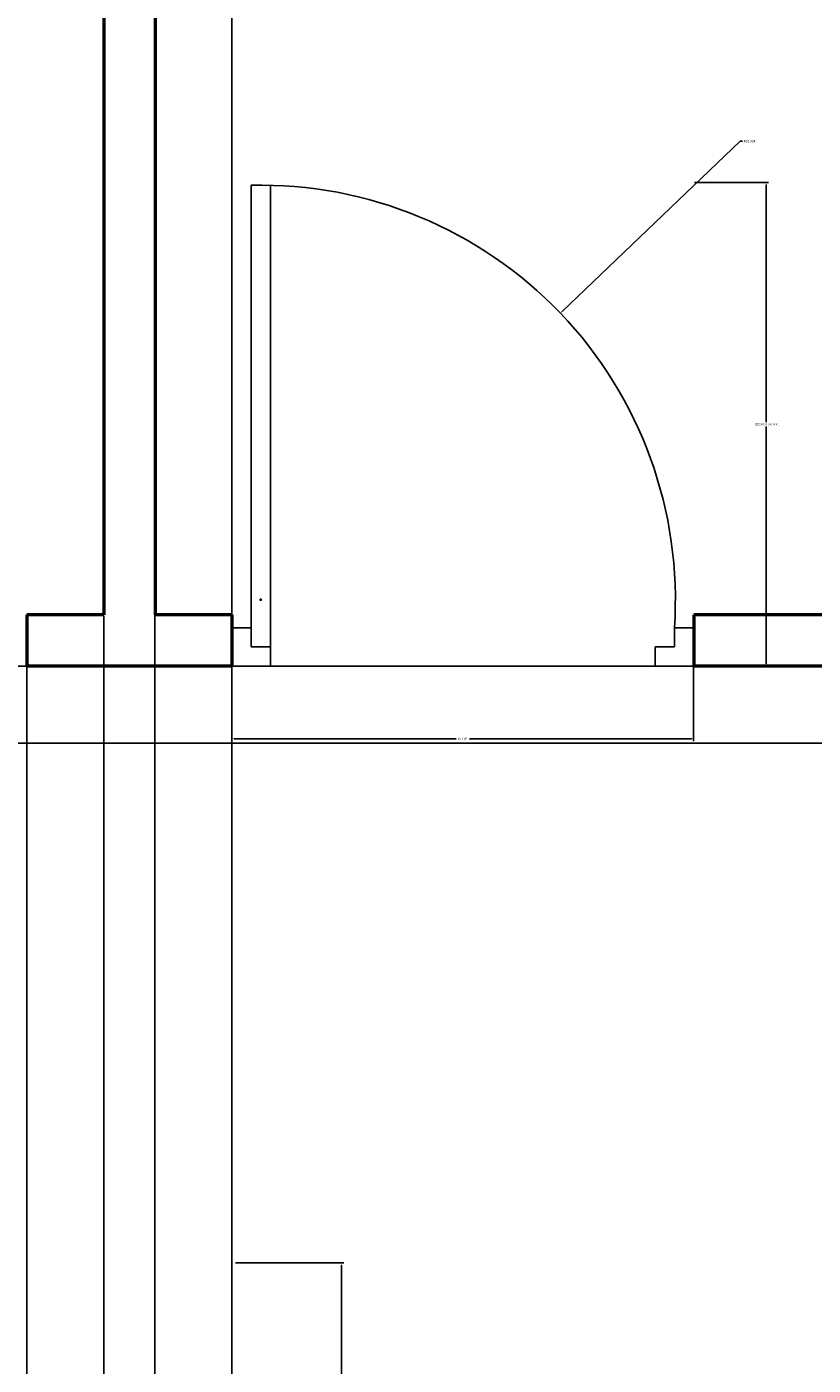
# Model space of a CAD drawing. Units: inches. Extents: x 1798 to 2141, y 1923 to 2386.
# Tile 7 of 9: x 1967 to 2028, y 2177 to 2281. Entities that reach past the tile are written whole.
import ezdxf

# ---------------------------------------------------------------- set-up
doc = ezdxf.new("R2010")
doc.units = ezdxf.units.IN
for name, color, linetype, lineweight in [('A-ANNO-DIMS', 2, 'Continuous', 18), ('A-FURN', 8, 'Continuous', 13), ('door', 40, 'Continuous', 25), ('wall', 4, 'Continuous', 50)]:
    doc.layers.add(name, color=color, linetype=linetype, lineweight=lineweight)
doc.styles.get("Standard").update_dxf_attribs({"font": 'arial.ttf'})
doc.dimstyles.get("Standard").update_dxf_attribs({"dimtxt": 0.18, "dimasz": 0.18, "dimexe": 0.18, "dimexo": 0.0625, "dimgap": 0.09, "dimtad": 0, "dimtih": 1, "dimtoh": 1, "dimdec": 4, "dimzin": 0, "dimdsep": 46, "dimtxsty": 'Standard', "dimcen": 0.09, "dimadec": 0, "dimazin": 0, "dimtfac": 1, "dimtdec": 4, "dimtofl": 0, "dimtmove": 0, "dimatfit": 3, "dimfxl": 1, "dimtolj": 1, "dimtzin": 0, "dimarcsym": 0})

# ---------------------------------------------------------------- blocks, each defined once
blk = doc.blocks.new('A$C45501D90')
for p, q in [((-242.2, 1133.5), (224, 1133.5)), ((-242.2, 1112.8), (-242.2, 1133.5)), ((224, 1112.8), (-242.2, 1112.8)), ((-242.2, 1111.2), (-202.3, 1079.2)), ((-156, 1109.6), (-132, 1085.6)), ((-108.1, 1109.6), (-84.1, 1085.6)), ((-60.2, 1109.6), (-36.2, 1085.6)), ((45.2, 1109.6), (21.2, 1085.6)), ((93.1, 1109.6), (69.1, 1085.6)), ((141, 1109.6), (117, 1085.6)), ((224, 1112.8), (187.3, 1079.2)), ((224, 1133.5), (224, 1112.8)), ((-203.9, 1106.4), (-165.6, 1108)), ((-168.8, 1080.8), (-203.9, 1106.4)), ((-202.3, 1079.2), (-168.8, 1080.8)), ((161.8, 1076.1), (-181.4, 1076.1)), ((-165.6, 1108), (-167.2, 1085.6)), ((-119.3, 1085.6), (-143.2, 1108)), ((-143.2, 1108), (-133.6, 1108)), ((-133.6, 1108), (-122.5, 1098.4)), ((-132, 1085.6), (-119.3, 1085.6)), ((-122.5, 1098.4), (-119.3, 1101.6)), ((-119.3, 1101.6), (-117.7, 1087.2)), ((-71.4, 1085.6), (-95.3, 1108)), ((-95.3, 1108), (-85.7, 1108)), ((-85.7, 1108), (-74.6, 1098.4)), ((-84.1, 1085.6), (-71.4, 1085.6)), ((-74.6, 1098.4), (-71.4, 1101.6)), ((-71.4, 1101.6), (-69.8, 1087.2)), ((-23.5, 1085.6), (-47.4, 1108)), ((-47.4, 1108), (-37.8, 1108)), ((-37.8, 1108), (-26.7, 1098.4)), ((-36.2, 1085.6), (-23.5, 1085.6)), ((-26.7, 1098.4), (-23.5, 1101.6)), ((-23.5, 1101.6), (-21.9, 1087.2)), ((8.5, 1101.6), (6.9, 1087.2)), ((8.5, 1085.6), (32.4, 1108)), ((11.6, 1098.4), (8.5, 1101.6)), ((21.2, 1085.6), (8.5, 1085.6)), ((22.8, 1108), (11.6, 1098.4)), ((32.4, 1108), (22.8, 1108)), ((56.3, 1101.6), (54.8, 1087.2)), ((56.3, 1085.6), (80.3, 1108)), ((59.5, 1098.4), (56.3, 1101.6)), ((69.1, 1085.6), (56.3, 1085.6)), ((70.7, 1108), (59.5, 1098.4)), ((80.3, 1108), (70.7, 1108)), ((104.2, 1101.6), (102.6, 1087.2)), ((104.2, 1085.6), (128.2, 1108)), ((107.4, 1098.4), (104.2, 1101.6)), ((117, 1085.6), (104.2, 1085.6)), ((118.6, 1108), (107.4, 1098.4)), ((128.2, 1108), (118.6, 1108)), ((188.9, 1106.4), (150.5, 1108)), ((150.5, 1108), (152.1, 1085.6)), ((153.7, 1080.8), (188.9, 1106.4)), ((187.3, 1079.2), (153.7, 1080.8)), ((-197.3, 1061.6), (-238.9, 627.6)), ((225.2, 627.8), (177.6, 1061.8)), ((842.6, 766.1), (860.5, 776.5)), ((860.5, 776.5), (1093.6, 372.8)), ((-1102.7, 357), (-869.7, 760.7)), ((-851.7, 750.4), (-1084.8, 346.6)), ((-869.7, 760.7), (-851.7, 750.4)), ((-848.7, 752.3), (-841, 701.8)), ((841.2, 765.3), (833.5, 714.8)), ((1075.7, 362.4), (842.6, 766.1)), ((851.7, 686.6), (856.2, 729.8)), ((856.2, 729.8), (876.7, 697.4)), ((-863.7, 716.7), (-884.3, 684.4)), ((-884.3, 684.4), (-864.1, 674.6)), ((-859.2, 673.6), (-863.7, 716.7)), ((-841, 701.8), (-859.2, 673.6)), ((-431.1, 509), (-830.8, 684.8)), ((820.7, 701.7), (424.1, 520.7)), ((833.5, 714.8), (851.7, 686.6)), ((1012.8, 397.9), (841.2, 695.1)), ((876.7, 697.4), (856.6, 687.6)), ((882.9, 689.9), (874.2, 657.2)), ((-851, 678.1), (-1022.6, 380.9)), ((-897.5, 642.2), (-901.9, 641.1)), ((-901.9, 641.1), (-890.2, 632.5)), ((-895.4, 665), (-900.2, 656.7)), ((-900.2, 656.7), (-897.5, 642.2)), ((-888.1, 633.1), (-895.4, 665)), ((-890.4, 676.9), (-881.7, 644.2)), ((-881.7, 644.2), (-888.1, 633.1)), ((874.2, 657.2), (880.6, 646.1)), ((880.6, 646.1), (887.9, 678)), ((894.4, 654.1), (882.7, 645.5)), ((887.9, 678), (892.7, 669.7)), ((892.7, 669.7), (890, 655.2)), ((890, 655.2), (894.4, 654.1)), ((906.9, 648.4), (898.1, 615.7)), ((-921.5, 600.8), (-925.8, 599.6)), ((-925.8, 599.6), (-914.2, 591)), ((-919.4, 623.5), (-924.2, 615.2)), ((-924.2, 615.2), (-921.5, 600.8)), ((-912, 591.6), (-919.4, 623.5)), ((-914.4, 635.4), (-905.6, 602.7)), ((-905.6, 602.7), (-912, 591.6)), ((-223, 610.1), (209.4, 610.1)), ((898.1, 615.7), (904.5, 604.6)), ((904.5, 604.6), (911.9, 636.5)), ((918.3, 612.6), (906.7, 604)), ((911.9, 636.5), (916.7, 628.2)), ((916.7, 628.2), (914, 613.8)), ((914, 613.8), (918.3, 612.6)), ((930.8, 606.9), (922.1, 574.2)), ((-945.4, 559.3), (-949.8, 558.1)), ((-949.8, 558.1), (-938.1, 549.6)), ((-943.3, 582), (-948.1, 573.8)), ((-948.1, 573.8), (-945.4, 559.3)), ((-936, 550.1), (-943.3, 582)), ((-938.3, 593.9), (-929.6, 561.2)), ((-929.6, 561.2), (-936, 550.1)), ((922.1, 574.2), (928.4, 563.1)), ((928.4, 563.1), (935.8, 595.1)), ((942.3, 571.1), (930.6, 562.6)), ((935.8, 595.1), (940.6, 586.8)), ((940.6, 586.8), (937.9, 572.3)), ((937.9, 572.3), (942.3, 571.1)), ((-951.9, 522.5), (-983.2, 512.9)), ((-983.2, 512.9), (-978.5, 521.2)), ((-978.5, 521.2), (-964.6, 526.1)), ((-964.6, 526.1), (-965.7, 530.5)), ((-965.7, 530.5), (-952.5, 524.7)), ((-958.3, 511.4), (-951.9, 522.5)), ((950.8, 524.4), (944.4, 535.5)), ((944.4, 535.5), (975.7, 525.9)), ((958.2, 543.5), (945, 537.7)), ((983.5, 515.7), (950.8, 524.4)), ((957.1, 539.1), (958.2, 543.5)), ((970.9, 534.2), (957.1, 539.1)), ((975.7, 525.9), (970.9, 534.2)), ((-1015, 461.2), (-982.3, 469.9)), ((-975.9, 481), (-1007.2, 471.4)), ((-1007.2, 471.4), (-1002.4, 479.7)), ((-1002.4, 479.7), (-988.5, 484.6)), ((-991, 502.7), (-958.3, 511.4)), ((-988.5, 484.6), (-989.7, 489)), ((-989.7, 489), (-976.5, 483.2)), ((-982.3, 469.9), (-975.9, 481)), ((-639.9, 111.9), (-423.7, 486.4)), ((-5.6, 508.7, 90.8), (0.4, 508.7, 90.8)), ((-5.6, 317.7, 90.8), (-5.6, 508.7, 90.8)), ((0.4, 508.7, 90.8), (0.4, 317.7, 90.8)), ((5.8, 317.7, 90.8), (5.8, 508.7, 90.8)), ((5.8, 508.7, 90.8), (11.8, 508.7, 90.8)), ((11.8, 508.7, 90.8), (11.8, 317.7, 90.8)), ((416.9, 498.2), (633.1, 123.7)), ((968.4, 494), (999.7, 484.4)), ((974.7, 483), (968.4, 494)), ((982.2, 502), (968.9, 496.2)), ((1007.4, 474.2), (974.7, 483)), ((981, 497.6), (982.2, 502)), ((994.9, 492.7), (981, 497.6)), ((999.7, 484.4), (994.9, 492.7)), ((-1038.9, 419.7), (-1006.2, 428.5)), ((-999.8, 439.5), (-1031.1, 430)), ((-1031.1, 430), (-1026.3, 438.3)), ((-1026.3, 438.3), (-1012.5, 443.1)), ((-1012.5, 443.1), (-1013.6, 447.5)), ((-1013.6, 447.5), (-1000.4, 441.7)), ((-1006.2, 428.5), (-999.8, 439.5)), ((998.7, 441.5), (992.3, 452.5)), ((992.3, 452.5), (1023.6, 443)), ((1006.1, 460.5), (992.9, 454.7)), ((1031.4, 432.7), (998.7, 441.5)), ((1005, 456.2), (1006.1, 460.5)), ((1018.8, 451.3), (1005, 456.2)), ((1023.6, 443), (1018.8, 451.3)), ((-1060.1, 376.6), (-1042.3, 410.6)), ((-1020.4, 394.3), (-1060.1, 376.6)), ((-1042.3, 410.6), (-1023.8, 398.1)), ((-1035.8, 364.4), (-1020.4, 394.3)), ((1028.3, 377.5), (1012.9, 407.3)), ((1012.9, 407.3), (1052.6, 389.6)), ((1034.8, 423.6), (1016.3, 411.1)), ((1052.6, 389.6), (1034.8, 423.6)), ((-1084.8, 346.6), (-1102.7, 357)), ((-1083.4, 345.8), (-1035.8, 364.4)), ((-1018, 360), (-663, 106.9)), ((-22.3, 329.1, 90.8), (-22.3, 344.6, 90.8)), ((-22.3, 344.6, 90.8), (-5.6, 344.6, 90.8)), ((0.4, 344.6, 90.8), (5.8, 344.6, 90.8)), ((11.8, 344.6, 90.8), (27.3, 344.6, 90.8)), ((27.3, 344.6, 90.8), (27.3, 329.1, 90.8)), ((656.3, 118.9), (1008.4, 377.1)), ((1075.9, 358.8), (1028.3, 377.5)), ((1093.6, 372.8), (1075.7, 362.4)), ((-5.6, 329.1, 90.8), (-22.3, 329.1, 90.8)), ((0.4, 317.7, 90.8), (-5.6, 317.7, 90.8)), ((5.8, 329.1, 90.8), (0.4, 329.1, 90.8)), ((11.8, 317.7, 90.8), (5.8, 317.7, 90.8)), ((27.3, 329.1, 90.8), (11.8, 329.1, 90.8)), ((-436.3, 265.3, 90.8), (-433.3, 270.5, 90.8)), ((-270.9, 169.9, 90.8), (-436.3, 265.3, 90.8)), ((-433.3, 270.5, 90.8), (-267.9, 175, 90.8)), ((-430.6, 275.2, 90.8), (-427.6, 280.3, 90.8)), ((-265.2, 179.7, 90.8), (-430.6, 275.2, 90.8)), ((-427.6, 280.3, 90.8), (-262.3, 184.9, 90.8)), ((-175.3, 276.1, 90.8), (-104.8, 293.2, 90.8)), ((-103.3, 252.4, 90.8), (-175.3, 276.1, 90.8)), ((-104.8, 293.2, 90.8), (-85.5, 278.4, 90.8)), ((-85.5, 278.4, 90.8), (-52.1, 293.9, 90.8)), ((9.5, 276.1, 90.8), (-59.5, 246.5, 90.8)), ((-52.1, 293.9, 90.8), (9.5, 276.1, 90.8)), ((134.3, 288, 90.8), (184.3, 235.5, 90.8)), ((149.7, 213.9, 90.8), (134.3, 288, 90.8)), ((255.2, 161.9, 90.8), (420.6, 257.3, 90.8)), ((420.6, 257.3, 90.8), (423.5, 252.2, 90.8)), ((-59.5, 246.5, 90.8), (-103.3, 252.4, 90.8)), ((166.5, 173, 90.8), (149.7, 213.9, 90.8)), ((184.3, 235.5, 90.8), (181.1, 211.4, 90.8)), ((423.5, 252.2, 90.8), (258.2, 156.7, 90.8)), ((260.9, 152, 90.8), (426.2, 247.5, 90.8)), ((429.2, 242.3, 90.8), (263.8, 146.9, 90.8)), ((426.2, 247.5, 90.8), (429.2, 242.3, 90.8)), ((-302.5, 168.8, 90.8), (-294.2, 183.3, 90.8)), ((-291.2, 188.5, 90.8), (-288.5, 193.1, 90.8)), ((-280.7, 175.5, 90.8), (-289.1, 161.1, 90.8)), ((-285.5, 198.3, 90.8), (-277.8, 211.7, 90.8)), ((-277.8, 211.7, 90.8), (-264.3, 204, 90.8)), ((-275.1, 185.4, 90.8), (-277.8, 180.7, 90.8)), ((-264.3, 204, 90.8), (-272.1, 190.5, 90.8)), ((-267.9, 175, 90.8), (-270.9, 169.9, 90.8)), ((-262.3, 184.9, 90.8), (-265.2, 179.7, 90.8)), ((226.7, 128.1, 90.8), (166.5, 173, 90.8)), ((181.1, 211.4, 90.8), (211.3, 190.3, 90.8)), ((211.3, 190.3, 90.8), (226.7, 128.1, 90.8)), ((256.6, 182, 90.8), (270.1, 189.8, 90.8)), ((265, 167.5, 90.8), (256.6, 182, 90.8)), ((270.1, 189.8, 90.8), (278.4, 175.3, 90.8)), ((-289.1, 161.1, 90.8), (-302.5, 168.8, 90.8)), ((-273.6, 117.6, 90.8), (-227.4, 162.1, 90.8)), ((-227.4, 162.1, 90.8), (-236.2, 87.5, 90.8)), ((258.2, 156.7, 90.8), (255.2, 161.9, 90.8)), ((263.8, 146.9, 90.8), (260.9, 152, 90.8)), ((270.7, 157.7, 90.8), (268, 162.4, 90.8)), ((281.4, 139.1, 90.8), (273.7, 152.5, 90.8)), ((281.4, 170.1, 90.8), (284.1, 165.5, 90.8)), ((294.9, 146.8, 90.8), (281.4, 139.1, 90.8)), ((287.1, 160.3, 90.8), (294.9, 146.8, 90.8)), ((-276.8, 80.9, 90.8), (-273.6, 117.6, 90.8)), ((-236.2, 87.5, 90.8), (-263.2, 52.5, 90.8)), ((-319.8, 2.1, 90.8), (-299.3, 71.7, 90.8)), ((-263.2, 52.5, 90.8), (-319.8, 2.1, 90.8)), ((-299.3, 71.7, 90.8), (-276.8, 80.9, 90.8)), ((242.9, -24.6, 90.8), (299.4, 25.9, 90.8)), ((299.4, 25.9, 90.8), (278.9, -43.7, 90.8)), ((215.8, -59.5, 90.8), (242.9, -24.6, 90.8)), ((207, -134.1, 90.8), (215.8, -59.5, 90.8)), ((256.4, -53, 90.8), (253.2, -89.7, 90.8)), ((278.9, -43.7, 90.8), (256.4, -53, 90.8)), ((-656.3, -118.9), (-1008.4, -377.1)), ((-416.9, -498.2), (-633.1, -123.7)), ((-449.6, -214.4, 90.8), (-284.2, -118.9, 90.8)), ((-281.2, -124.1, 90.8), (-446.6, -219.5, 90.8)), ((-315.2, -118.9, 90.8), (-301.8, -111.1, 90.8)), ((-307.5, -132.3, 90.8), (-315.2, -118.9, 90.8)), ((-301.8, -111.1, 90.8), (-294, -124.6, 90.8)), ((-284.2, -118.9, 90.8), (-281.2, -124.1, 90.8)), ((-247, -100.1, 90.8), (-186.8, -145, 90.8)), ((-231.7, -162.3, 90.8), (-247, -100.1, 90.8)), ((253.2, -89.7, 90.8), (207, -134.1, 90.8)), ((639.9, -111.9), (423.7, -486.4)), ((1018, -360), (663, -106.9)), ((-443.9, -224.2, 90.8), (-278.5, -128.7, 90.8)), ((-275.5, -133.9, 90.8), (-440.9, -229.4, 90.8)), ((-301.8, -142.1, 90.8), (-304.5, -137.5, 90.8)), ((-290.4, -161.8, 90.8), (-298.8, -147.3, 90.8)), ((-291, -129.7, 90.8), (-288.3, -134.4, 90.8)), ((-277, -154, 90.8), (-290.4, -161.8, 90.8)), ((-285.4, -139.5, 90.8), (-277, -154, 90.8)), ((-278.5, -128.7, 90.8), (-275.5, -133.9, 90.8)), ((-201.5, -183.4, 90.8), (-231.7, -162.3, 90.8)), ((-186.8, -145, 90.8), (-170.1, -185.9, 90.8)), ((241.9, -156.9, 90.8), (244.9, -151.7, 90.8)), ((407.3, -252.4, 90.8), (241.9, -156.9, 90.8)), ((244, -176, 90.8), (251.7, -162.5, 90.8)), ((244.9, -151.7, 90.8), (410.3, -247.2, 90.8)), ((247.6, -147.1, 90.8), (250.6, -141.9, 90.8)), ((413, -242.5, 90.8), (247.6, -147.1, 90.8)), ((250.6, -141.9, 90.8), (415.9, -237.4, 90.8)), ((254.7, -157.4, 90.8), (257.4, -152.7, 90.8)), ((265.2, -170.3, 90.8), (257.4, -183.7, 90.8)), ((260.4, -147.6, 90.8), (268.7, -133.1, 90.8)), ((270.8, -160.5, 90.8), (268.1, -165.1, 90.8)), ((268.7, -133.1, 90.8), (282.2, -140.8, 90.8)), ((282.2, -140.8, 90.8), (273.8, -155.3, 90.8)), ((-204.7, -207.6, 90.8), (-201.5, -183.4, 90.8)), ((-154.7, -260.1, 90.8), (-204.7, -207.6, 90.8)), ((-170.1, -185.9, 90.8), (-154.7, -260.1, 90.8)), ((257.4, -183.7, 90.8), (244, -176, 90.8)), ((-446.6, -219.5, 90.8), (-449.6, -214.4, 90.8)), ((-440.9, -229.4, 90.8), (-443.9, -224.2, 90.8)), ((-29.8, -248.2, 90.8), (39.2, -218.5, 90.8)), ((31.8, -266, 90.8), (-29.8, -248.2, 90.8)), ((65.2, -250.4, 90.8), (31.8, -266, 90.8)), ((39.2, -218.5, 90.8), (83, -224.4, 90.8)), ((84.4, -265.2, 90.8), (65.2, -250.4, 90.8)), ((83, -224.4, 90.8), (154.9, -248.2, 90.8)), ((154.9, -248.2, 90.8), (84.4, -265.2, 90.8)), ((410.3, -247.2, 90.8), (407.3, -252.4, 90.8)), ((415.9, -237.4, 90.8), (413, -242.5, 90.8)), ((-32.1, -480.7, 90.8), (-32.1, -289.8, 90.8)), ((-32.1, -289.8, 90.8), (-26.1, -289.8, 90.8)), ((-26.1, -289.8, 90.8), (-26.1, -480.7, 90.8)), ((-20.8, -480.7, 90.8), (-20.8, -289.8, 90.8)), ((-20.8, -289.8, 90.8), (-14.8, -289.8, 90.8)), ((-14.8, -289.8, 90.8), (-14.8, -480.7, 90.8)), ((-47.6, -316.6, 90.8), (-47.6, -301.1, 90.8)), ((-47.6, -301.1, 90.8), (-32.1, -301.1, 90.8)), ((-32.1, -316.6, 90.8), (-47.6, -316.6, 90.8)), ((-26.1, -301.1, 90.8), (-20.8, -301.1, 90.8)), ((-20.8, -316.6, 90.8), (-26.1, -316.6, 90.8)), ((-14.8, -301.1, 90.8), (1.9, -301.1, 90.8)), ((1.9, -316.6, 90.8), (-14.8, -316.6, 90.8)), ((1.9, -301.1, 90.8), (1.9, -316.6, 90.8)), ((-1093.6, -372.8), (-1075.7, -362.4)), ((-860.5, -776.5), (-1093.6, -372.8)), ((-1075.9, -358.8), (-1028.3, -377.5)), ((-1075.7, -362.4), (-842.6, -766.1)), ((-1028.3, -377.5), (-1012.9, -407.3)), ((851, -678.1), (1022.6, -380.9)), ((851.7, -750.4), (1084.8, -346.6)), ((1102.7, -357), (869.7, -760.7)), ((1035.8, -364.4), (1020.4, -394.3)), ((1020.4, -394.3), (1060.1, -376.6)), ((1083.4, -345.8), (1035.8, -364.4)), ((1060.1, -376.6), (1042.3, -410.6)), ((1084.8, -346.6), (1102.7, -357)), ((-1052.6, -389.6), (-1034.8, -423.6)), ((-1012.9, -407.3), (-1052.6, -389.6)), ((-1034.8, -423.6), (-1016.3, -411.1)), ((-1012.8, -397.9), (-841.2, -695.1)), ((1038.9, -419.7), (1006.2, -428.5)), ((1042.3, -410.6), (1023.8, -398.1)), ((-1031.4, -432.7), (-998.7, -441.5)), ((-1023.6, -443), (-1018.8, -451.3)), ((-992.3, -452.5), (-1023.6, -443)), ((-1018.8, -451.3), (-1005, -456.2)), ((-1006.1, -460.5), (-992.9, -454.7)), ((-1005, -456.2), (-1006.1, -460.5)), ((-998.7, -441.5), (-992.3, -452.5)), ((1015, -461.2), (982.3, -469.9)), ((1006.2, -428.5), (999.8, -439.5)), ((999.8, -439.5), (1031.1, -430)), ((1013.6, -447.5), (1000.4, -441.7)), ((1026.3, -438.3), (1012.5, -443.1)), ((1012.5, -443.1), (1013.6, -447.5)), ((1031.1, -430), (1026.3, -438.3)), ((-1007.4, -474.2), (-974.7, -483)), ((-968.4, -494), (-999.7, -484.4)), ((-999.7, -484.4), (-994.9, -492.7)), ((-994.9, -492.7), (-981, -497.6)), ((-982.2, -502), (-968.9, -496.2)), ((-981, -497.6), (-982.2, -502)), ((-974.7, -483), (-968.4, -494)), ((-26.1, -480.7, 90.8), (-32.1, -480.7, 90.8)), ((-14.8, -480.7, 90.8), (-20.8, -480.7, 90.8)), ((431.1, -509), (830.8, -684.8)), ((958.3, -511.4), (951.9, -522.5)), ((991, -502.7), (958.3, -511.4)), ((982.3, -469.9), (975.9, -481)), ((975.9, -481), (1007.2, -471.4)), ((989.7, -489), (976.5, -483.2)), ((1002.4, -479.7), (988.5, -484.6)), ((988.5, -484.6), (989.7, -489)), ((1007.2, -471.4), (1002.4, -479.7)), ((-983.5, -515.7), (-950.8, -524.4)), ((-944.4, -535.5), (-975.7, -525.9)), ((-975.7, -525.9), (-970.9, -534.2)), ((-970.9, -534.2), (-957.1, -539.1)), ((-958.2, -543.5), (-945, -537.7)), ((-957.1, -539.1), (-958.2, -543.5)), ((-950.8, -524.4), (-944.4, -535.5)), ((-820.7, -701.7), (-424.1, -520.7)), ((929.6, -561.2), (936, -550.1)), ((936, -550.1), (943.3, -582)), ((949.8, -558.1), (938.1, -549.6)), ((951.9, -522.5), (983.2, -512.9)), ((965.7, -530.5), (952.5, -524.7)), ((978.5, -521.2), (964.6, -526.1)), ((964.6, -526.1), (965.7, -530.5)), ((983.2, -512.9), (978.5, -521.2)), ((-942.3, -571.1), (-930.6, -562.6)), ((-937.9, -572.3), (-942.3, -571.1)), ((-940.6, -586.8), (-937.9, -572.3)), ((-935.8, -595.1), (-940.6, -586.8)), ((-928.4, -563.1), (-935.8, -595.1)), ((-930.8, -606.9), (-922.1, -574.2)), ((-922.1, -574.2), (-928.4, -563.1)), ((905.6, -602.7), (912, -591.6)), ((912, -591.6), (919.4, -623.5)), ((925.8, -599.6), (914.2, -591)), ((938.3, -593.9), (929.6, -561.2)), ((943.3, -582), (948.1, -573.8)), ((945.4, -559.3), (949.8, -558.1)), ((948.1, -573.8), (945.4, -559.3)), ((-918.3, -612.6), (-906.7, -604)), ((-914, -613.8), (-918.3, -612.6)), ((-916.7, -628.2), (-914, -613.8)), ((-911.9, -636.5), (-916.7, -628.2)), ((-904.5, -604.6), (-911.9, -636.5)), ((-906.9, -648.4), (-898.1, -615.7)), ((-898.1, -615.7), (-904.5, -604.6)), ((-229.3, -629.3), (-181.8, -1063.3)), ((-225.2, -627.8), (-177.6, -1061.8)), ((218.9, -611.6), (-213.5, -611.6)), ((223, -610.1), (-209.4, -610.1)), ((193.2, -1063.1), (234.8, -629.1)), ((197.3, -1061.6), (238.9, -627.6)), ((881.7, -644.2), (888.1, -633.1)), ((888.1, -633.1), (895.4, -665)), ((901.9, -641.1), (890.2, -632.5)), ((914.4, -635.4), (905.6, -602.7)), ((919.4, -623.5), (924.2, -615.2)), ((921.5, -600.8), (925.8, -599.6)), ((924.2, -615.2), (921.5, -600.8)), ((-894.4, -654.1), (-882.7, -645.5)), ((-890, -655.2), (-894.4, -654.1)), ((-892.7, -669.7), (-890, -655.2)), ((-887.9, -678), (-892.7, -669.7)), ((-880.6, -646.1), (-887.9, -678)), ((-882.9, -689.9), (-874.2, -657.2)), ((-874.2, -657.2), (-880.6, -646.1)), ((841, -701.8), (859.2, -673.6)), ((859.2, -673.6), (863.7, -716.7)), ((884.3, -684.4), (864.1, -674.6)), ((890.4, -676.9), (881.7, -644.2)), ((895.4, -665), (900.2, -656.7)), ((897.5, -642.2), (901.9, -641.1)), ((900.2, -656.7), (897.5, -642.2)), ((-876.7, -697.4), (-856.6, -687.6)), ((-856.2, -729.8), (-876.7, -697.4)), ((-851.7, -686.6), (-856.2, -729.8)), ((-833.5, -714.8), (-851.7, -686.6)), ((-841.2, -765.3), (-833.5, -714.8)), ((848.7, -752.3), (841, -701.8)), ((863.7, -716.7), (884.3, -684.4)), ((-842.6, -766.1), (-860.5, -776.5)), ((869.7, -760.7), (851.7, -750.4)), ((-231.3, -1112.7), (-191.4, -1080.8)), ((-227.2, -1111.2), (-187.3, -1079.2)), ((-157.9, -1082.4), (-193, -1107.9)), ((-193, -1107.9), (-154.7, -1109.5)), ((-191.4, -1080.8), (-157.9, -1082.4)), ((-153.7, -1080.8), (-188.9, -1106.4)), ((-188.9, -1106.4), (-150.5, -1108)), ((-187.3, -1079.2), (-153.7, -1080.8)), ((-165.9, -1077.6), (177.3, -1077.6)), ((-161.8, -1076.1), (181.4, -1076.1)), ((-154.7, -1109.5), (-156.3, -1087.1)), ((-150.5, -1108), (-152.1, -1085.6)), ((-145.1, -1111.1), (-121.1, -1087.1)), ((-141, -1109.6), (-117, -1085.6)), ((-108.4, -1087.1), (-132.3, -1109.5)), ((-104.2, -1085.6), (-128.2, -1108)), ((-128.2, -1108), (-118.6, -1108)), ((-122.7, -1109.5), (-111.6, -1099.9)), ((-121.1, -1087.1), (-108.4, -1087.1)), ((-118.6, -1108), (-107.4, -1098.4)), ((-117, -1085.6), (-104.2, -1085.6)), ((-111.6, -1099.9), (-108.4, -1103.1)), ((-108.4, -1103.1), (-106.8, -1088.7)), ((-107.4, -1098.4), (-104.2, -1101.6)), ((-104.2, -1101.6), (-102.6, -1087.2)), ((-97.2, -1111.1), (-73.2, -1087.1)), ((-93.1, -1109.6), (-69.1, -1085.6)), ((-60.5, -1087.1), (-84.4, -1109.5)), ((-56.3, -1085.6), (-80.3, -1108)), ((-80.3, -1108), (-70.7, -1108)), ((-74.8, -1109.5), (-63.7, -1099.9)), ((-73.2, -1087.1), (-60.5, -1087.1)), ((-70.7, -1108), (-59.5, -1098.4)), ((-69.1, -1085.6), (-56.3, -1085.6)), ((-63.7, -1099.9), (-60.5, -1103.1)), ((-60.5, -1103.1), (-58.9, -1088.7)), ((-59.5, -1098.4), (-56.3, -1101.6)), ((-56.3, -1101.6), (-54.8, -1087.2)), ((-49.3, -1111.1), (-25.3, -1087.1)), ((-45.2, -1109.6), (-21.2, -1085.6)), ((-12.6, -1087.1), (-36.5, -1109.5)), ((-8.5, -1085.6), (-32.4, -1108)), ((-32.4, -1108), (-22.8, -1108)), ((-26.9, -1109.5), (-15.8, -1099.9)), ((-25.3, -1087.1), (-12.6, -1087.1)), ((-22.8, -1108), (-11.6, -1098.4)), ((-21.2, -1085.6), (-8.5, -1085.6)), ((-15.8, -1099.9), (-12.6, -1103.1)), ((-12.6, -1103.1), (-11, -1088.7)), ((-11.6, -1098.4), (-8.5, -1101.6)), ((-8.5, -1101.6), (-6.9, -1087.2)), ((19.4, -1103.1), (17.8, -1088.7)), ((19.4, -1087.1), (43.3, -1109.5)), ((32.1, -1087.1), (19.4, -1087.1)), ((22.6, -1099.9), (19.4, -1103.1)), ((23.5, -1101.6), (21.9, -1087.2)), ((33.7, -1109.5), (22.6, -1099.9)), ((23.5, -1085.6), (47.4, -1108)), ((36.2, -1085.6), (23.5, -1085.6)), ((26.7, -1098.4), (23.5, -1101.6)), ((37.8, -1108), (26.7, -1098.4)), ((56.1, -1111.1), (32.1, -1087.1)), ((60.2, -1109.6), (36.2, -1085.6)), ((47.4, -1108), (37.8, -1108)), ((67.3, -1103.1), (65.7, -1088.7)), ((67.3, -1087.1), (91.2, -1109.5)), ((80, -1087.1), (67.3, -1087.1)), ((70.4, -1099.9), (67.3, -1103.1)), ((71.4, -1101.6), (69.8, -1087.2)), ((81.6, -1109.5), (70.4, -1099.9)), ((71.4, -1085.6), (95.3, -1108)), ((84.1, -1085.6), (71.4, -1085.6)), ((74.6, -1098.4), (71.4, -1101.6)), ((85.7, -1108), (74.6, -1098.4)), ((104, -1111.1), (80, -1087.1)), ((108.1, -1109.6), (84.1, -1085.6)), ((95.3, -1108), (85.7, -1108)), ((115.1, -1103.1), (113.6, -1088.7)), ((115.1, -1087.1), (139.1, -1109.5)), ((127.9, -1087.1), (115.1, -1087.1)), ((118.3, -1099.9), (115.1, -1103.1)), ((119.3, -1101.6), (117.7, -1087.2)), ((129.5, -1109.5), (118.3, -1099.9)), ((119.3, -1085.6), (143.2, -1108)), ((132, -1085.6), (119.3, -1085.6)), ((122.5, -1098.4), (119.3, -1101.6)), ((133.6, -1108), (122.5, -1098.4)), ((151.9, -1111.1), (127.9, -1087.1)), ((156, -1109.6), (132, -1085.6)), ((143.2, -1108), (133.6, -1108)), ((161.4, -1109.5), (163, -1087.1)), ((199.8, -1107.9), (161.4, -1109.5)), ((198.2, -1080.8), (164.6, -1082.4)), ((164.6, -1082.4), (199.8, -1107.9)), ((165.6, -1108), (167.2, -1085.6)), ((203.9, -1106.4), (165.6, -1108)), ((202.3, -1079.2), (168.8, -1080.8)), ((168.8, -1080.8), (203.9, -1106.4)), ((238.1, -1112.7), (198.2, -1080.8)), ((242.2, -1111.2), (202.3, -1079.2)), ((-228.1, -1114.3), (238.1, -1114.3)), ((-228.1, -1135), (-228.1, -1114.3)), ((238.1, -1135), (-228.1, -1135)), ((-224, -1112.8), (242.2, -1112.8)), ((-224, -1133.5), (-224, -1112.8)), ((242.2, -1133.5), (-224, -1133.5)), ((-132.3, -1109.5), (-122.7, -1109.5)), ((-84.4, -1109.5), (-74.8, -1109.5)), ((-36.5, -1109.5), (-26.9, -1109.5)), ((43.3, -1109.5), (33.7, -1109.5)), ((91.2, -1109.5), (81.6, -1109.5)), ((139.1, -1109.5), (129.5, -1109.5)), ((238.1, -1114.3), (238.1, -1135)), ((242.2, -1112.8), (242.2, -1133.5))]:
    blk.add_line(p, q)
for centre, radius in [((0, 0), 537), ((0, 0), 527), ((-94.8, 394.7, 90.8), 61.3), ((96.9, 390, 90.8), 56.9), ((95.5, 390.7, 90.8), 29.4), ((-282.3, 294.7, 90.8), 56.9), ((-283.5, 293.9, 90.8), 29.4), ((277.2, 277.6, 90.8), 61.3), ((-382.1, 131.1, 90.8), 61.3), ((369, 109.3, 90.8), 56.9), ((368.9, 110.8, 90.8), 29.4), ((-389.3, -81.3, 90.8), 56.9), ((361.8, -103.1, 90.8), 61.3), ((-389.2, -82.8, 90.8), 29.4), ((-297.5, -249.6, 90.8), 61.3), ((261.9, -266.7, 90.8), 56.9), ((263.2, -265.9, 90.8), 29.4), ((-117.2, -362, 90.8), 56.9), ((-115.9, -362.7, 90.8), 29.4), ((74.4, -366.7, 90.8), 61.3)]:
    blk.add_circle(centre, radius)
for centre, radius, start, end in [((-181.4, 1060.1), 16, 90, 174.5199), ((161.8, 1060.1), 16, 6.2572, 90), ((-837.2, 670.1), 16, 66.2572, 150), ((827.4, 687.1), 16, 30, 114.5199), ((-223, 626.1), 16, 174.5199, 270), ((209.4, 626.1), 16, 270, 6.2572), ((430.7, 506.2), 16, 114.5199, 210), ((-437.5, 494.4), 16, 330, 66.2572), ((999, 389.9), 16, 306.2572, 30), ((-1008.8, 373), 16, 150, 234.5199), ((-77.3, 270.2, 90.8), 44.6, 25.8558, 153.3359), ((-77.3, 270.2, 90.8), 44.6, 195.9338, 342.9389), ((178.1, 200.3, 90.8), 44.6, 135.9338, 282.9389), ((178.1, 200.3, 90.8), 44.6, 325.8558, 93.3359), ((-265.7, 83.9, 90.8), 44.6, 85.8558, 213.3359), ((-653.7, 119.9), 16, 234.5199, 330), ((-265.7, 83.9, 90.8), 44.6, 255.9338, 42.9389), ((646.9, 131.7), 16, 210, 306.2572), ((245.3, -55.9, 90.8), 44.6, 75.9338, 222.9389), ((245.3, -55.9, 90.8), 44.6, 265.8558, 33.3359), ((-646.9, -131.7), 16, 30, 126.2572), ((-198.5, -172.3, 90.8), 44.6, 315.9338, 102.9389), ((653.7, -119.9), 16, 54.5199, 150), ((-198.5, -172.3, 90.8), 44.6, 145.8558, 273.3359), ((57, -242.2, 90.8), 44.6, 15.9338, 162.9389), ((57, -242.2, 90.8), 44.6, 205.8558, 333.3359), ((-999, -389.9), 16, 126.2572, 210), ((1008.8, -373), 16, 330, 54.5199), ((-430.7, -506.2), 16, 294.5199, 30), ((437.5, -494.4), 16, 150, 246.2572), ((-213.5, -627.6), 16, 90, 186.2572), ((-209.4, -626.1), 16, 90, 186.2572), ((218.9, -627.6), 16, 354.5199, 90), ((223, -626.1), 16, 354.5199, 90), ((837.2, -670.1), 16, 246.2572, 330), ((-827.4, -687.1), 16, 210, 294.5199), ((-165.9, -1061.6), 16, 186.2572, 270), ((-161.8, -1060.1), 16, 186.2572, 270), ((177.3, -1061.6), 16, 270, 354.5199), ((181.4, -1060.1), 16, 270, 354.5199)]:
    blk.add_arc(centre, radius, start, end)
blk = doc.blocks.new('DOOR-SWING-36IN')
for p, q in [((1.5, 1.5), (1.5, 37.5)), ((3, 1.5), (3, 37.5)), ((0, 3), (0, 0)), ((1.5, 3), (0, 3)), ((1.5, 1.5), (1.5, 3)), ((34.5, 1.5), (34.5, 3)), ((34.5, 3), (36, 3)), ((36, 3), (36, 0)), ((3, 1.5), (1.5, 1.5)), ((3, 0), (3, 1.5)), ((33, 0), (33, 1.5)), ((33, 1.5), (34.5, 1.5)), ((0, 0), (3, 0)), ((36, 0), (33, 0))]:
    blk.add_line(p, q)
blk.add_arc((2.25, 5.18), 32.32, 356.1244, 91.3295)
blk = doc.blocks.new('*D19')
at = {"layer": 'A-ANNO-DIMS', "color": 0, "lineweight": -2, "transparency": 16777216}
for p, q in [((2018.58, 2269.03), (2024.35, 2269.03)), ((2024.17, 2268.85), (2024.17, 2250.36)), ((2024.17, 2231.5), (2024.17, 2250)), ((2018.58, 2231.32), (2024.35, 2231.32))]:
    blk.add_line(p, q, dxfattribs=at)
at = {"layer": 'A-ANNO-DIMS', "color": 0, "transparency": 16777216}
for points in [[(2024.14, 2268.85), (2024.2, 2268.85), (2024.17, 2269.03)], [(2024.14, 2231.5), (2024.2, 2231.5), (2024.17, 2231.32)]]:
    blk.add_solid(points, dxfattribs=at)
at = {"layer": 'Defpoints', "color": 0, "transparency": 16777216}
for p in [(2018.51, 2269.03), (2024.17, 2269.03), (2018.51, 2231.32)]:
    blk.add_point(p, dxfattribs=at)
at = {"layer": 'A-ANNO-DIMS', "color": 0, "transparency": 16777216, "insert": (2024.17, 2250.18), "char_height": 0.18, "attachment_point": 5}
blk.add_mtext('\\A1;DOOR D1 38 TYP.', dxfattribs=at)
blk = doc.blocks.new('*D20')
at = {"layer": 'A-ANNO-DIMS', "color": 0, "lineweight": -2, "transparency": 16777216}
for p, q in [((1982.51, 2231.26), (1982.51, 2225.49)), ((2018.51, 2231.26), (2018.51, 2225.49)), ((1982.69, 2225.67), (1999.99, 2225.67)), ((2018.33, 2225.67), (2001.04, 2225.67))]:
    blk.add_line(p, q, dxfattribs=at)
at = {"layer": 'A-ANNO-DIMS', "color": 0, "transparency": 16777216}
for points in [[(1982.69, 2225.7), (1982.69, 2225.64), (1982.51, 2225.67)], [(2018.33, 2225.7), (2018.33, 2225.64), (2018.51, 2225.67)]]:
    blk.add_solid(points, dxfattribs=at)
at = {"layer": 'Defpoints', "color": 0, "transparency": 16777216}
for p in [(1982.51, 2231.32), (2018.51, 2231.32), (2018.51, 2225.67)]:
    blk.add_point(p, dxfattribs=at)
at = {"layer": 'A-ANNO-DIMS', "color": 0, "transparency": 16777216, "insert": (2000.51, 2225.67), "char_height": 0.18, "attachment_point": 5}
blk.add_mtext('\\A1;36 TYP.', dxfattribs=at)
blk = doc.blocks.new('*D23')
at = {"layer": 'A-ANNO-DIMS', "color": 0, "lineweight": -2, "transparency": 16777216}
for p, q in [((1982.78, 2184.81), (1991.23, 2184.81)), ((1991.05, 2184.63), (1991.05, 2157.25)), ((1991.05, 2129.5), (1991.05, 2156.88)), ((1982.78, 2129.32), (1991.23, 2129.32))]:
    blk.add_line(p, q, dxfattribs=at)
at = {"layer": 'A-ANNO-DIMS', "color": 0, "transparency": 16777216}
for points in [[(1991.02, 2184.63), (1991.08, 2184.63), (1991.05, 2184.81)], [(1991.02, 2129.5), (1991.08, 2129.5), (1991.05, 2129.32)]]:
    blk.add_solid(points, dxfattribs=at)
at = {"layer": 'Defpoints', "color": 0, "transparency": 16777216}
for p in [(1982.72, 2184.81), (1991.05, 2184.81), (1982.72, 2129.32)]:
    blk.add_point(p, dxfattribs=at)
at = {"layer": 'A-ANNO-DIMS', "color": 0, "transparency": 16777216, "insert": (1991.05, 2157.07), "char_height": 0.18, "attachment_point": 5}
blk.add_mtext('\\A1;DINING SET 55', dxfattribs=at)
blk = doc.blocks.new('*D35')
at = {"layer": 'A-ANNO-DIMS', "color": 0, "lineweight": -2, "transparency": 16777216}
for p, q in [((1972.51, 2235.26), (1972.51, 1923.12)), ((1966.51, 2231.26), (1966.51, 1923.12)), ((1966.69, 1923.3), (1969.36, 1923.3)), ((1972.33, 1923.3), (1969.66, 1923.3))]:
    blk.add_line(p, q, dxfattribs=at)
at = {"layer": 'A-ANNO-DIMS', "color": 0, "transparency": 16777216}
for points in [[(1966.69, 1923.33), (1966.69, 1923.27), (1966.51, 1923.3)], [(1972.33, 1923.33), (1972.33, 1923.27), (1972.51, 1923.3)]]:
    blk.add_solid(points, dxfattribs=at)
at = {"layer": 'Defpoints', "color": 0, "transparency": 16777216}
for p in [(1972.51, 2235.32), (1966.51, 2231.32), (1972.51, 1923.3)]:
    blk.add_point(p, dxfattribs=at)
at = {"layer": 'A-ANNO-DIMS', "color": 0, "transparency": 16777216, "insert": (1969.51, 1923.3), "char_height": 0.18, "attachment_point": 5}
blk.add_mtext('\\A1;6', dxfattribs=at)
blk = doc.blocks.new('*D36')
at = {"layer": 'A-ANNO-DIMS', "color": 0, "lineweight": -2, "transparency": 16777216}
for p, q in [((1976.51, 2231.26), (1976.51, 1923.12)), ((1982.51, 2231.26), (1982.51, 1923.12)), ((1976.69, 1923.3), (1979.36, 1923.3)), ((1982.33, 1923.3), (1979.66, 1923.3))]:
    blk.add_line(p, q, dxfattribs=at)
at = {"layer": 'A-ANNO-DIMS', "color": 0, "transparency": 16777216}
for points in [[(1976.69, 1923.33), (1976.69, 1923.27), (1976.51, 1923.3)], [(1982.33, 1923.33), (1982.33, 1923.27), (1982.51, 1923.3)]]:
    blk.add_solid(points, dxfattribs=at)
at = {"layer": 'Defpoints', "color": 0, "transparency": 16777216}
for p in [(1976.51, 2231.32), (1982.51, 2231.32), (1982.51, 1923.3)]:
    blk.add_point(p, dxfattribs=at)
at = {"layer": 'A-ANNO-DIMS', "color": 0, "transparency": 16777216, "insert": (1979.51, 1923.3), "char_height": 0.18, "attachment_point": 5}
blk.add_mtext('\\A1;6', dxfattribs=at)
blk = doc.blocks.new('*D37')
at = {"layer": 'A-ANNO-DIMS', "color": 0, "lineweight": -2, "transparency": 16777216}
for p, q in [((2034.45, 2231.32), (1798.31, 2231.32)), ((1798.49, 2231.14), (1798.49, 2228.51)), ((1798.49, 2225.5), (1798.49, 2228.14)), ((2034.45, 2225.32), (1798.31, 2225.32))]:
    blk.add_line(p, q, dxfattribs=at)
at = {"layer": 'A-ANNO-DIMS', "color": 0, "transparency": 16777216}
for points in [[(1798.46, 2231.14), (1798.52, 2231.14), (1798.49, 2231.32)], [(1798.46, 2225.5), (1798.52, 2225.5), (1798.49, 2225.32)]]:
    blk.add_solid(points, dxfattribs=at)
at = {"layer": 'Defpoints', "color": 0, "transparency": 16777216}
for p in [(1798.49, 2231.32), (2034.51, 2231.32), (2034.51, 2225.32)]:
    blk.add_point(p, dxfattribs=at)
at = {"layer": 'A-ANNO-DIMS', "color": 0, "transparency": 16777216, "insert": (1798.49, 2228.32), "char_height": 0.18, "attachment_point": 5}
blk.add_mtext('\\A1;6', dxfattribs=at)
blk = doc.blocks.new('*D39')
at = {"layer": 'A-ANNO-DIMS', "color": 0, "lineweight": -2, "transparency": 16777216}
for p, q in [((1976.51, 2035.39), (1976.51, 2385.53)), ((1982.51, 2035.39), (1982.51, 2385.53)), ((1976.69, 2385.35), (1979.36, 2385.35)), ((1982.33, 2385.35), (1979.66, 2385.35))]:
    blk.add_line(p, q, dxfattribs=at)
at = {"layer": 'A-ANNO-DIMS', "color": 0, "transparency": 16777216}
for points in [[(1976.69, 2385.38), (1976.69, 2385.32), (1976.51, 2385.35)], [(1982.33, 2385.38), (1982.33, 2385.32), (1982.51, 2385.35)]]:
    blk.add_solid(points, dxfattribs=at)
at = {"layer": 'Defpoints', "color": 0, "transparency": 16777216}
for p in [(1982.51, 2385.35), (1976.51, 2035.32), (1982.51, 2035.32)]:
    blk.add_point(p, dxfattribs=at)
at = {"layer": 'A-ANNO-DIMS', "color": 0, "transparency": 16777216, "insert": (1979.51, 2385.35), "char_height": 0.18, "attachment_point": 5}
blk.add_mtext('\\A1;6', dxfattribs=at)
blk = doc.blocks.new('*D51')
at = {"layer": 'A-ANNO-DIMS', "color": 0, "lineweight": -2, "transparency": 16777216}
for p, q in [((2022.14, 2272.26), (2008.25, 2258.98)), ((2022.32, 2272.26), (2022.14, 2272.26)), ((1984.67, 2236.51), (1984.85, 2236.51)), ((1984.76, 2236.42), (1984.76, 2236.6))]:
    blk.add_line(p, q, dxfattribs=at)
at = {"layer": 'A-ANNO-DIMS', "color": 0, "transparency": 16777216}
blk.add_solid([(2008.23, 2259), (2008.27, 2258.95), (2008.12, 2258.85)], dxfattribs=at)
at = {"layer": 'Defpoints', "color": 0, "transparency": 16777216}
for p in [(2008.12, 2258.85), (1984.76, 2236.51)]:
    blk.add_point(p, dxfattribs=at)
at = {"layer": 'A-ANNO-DIMS', "color": 0, "transparency": 16777216, "insert": (2022.87, 2272.26), "char_height": 0.18, "attachment_point": 5}
blk.add_mtext('\\A1;R32.324', dxfattribs=at)

msp = doc.modelspace()

# ---------------------------------------------------------------- linework, layer by layer
at = {"layer": 'wall'}
for p, q in [((1972.5141, 2355.3239), (1972.5141, 2235.3239)), ((1976.5141, 2355.3239), (1976.5141, 2235.3239)), ((1972.5141, 2235.3239), (1966.5141, 2235.3239)), ((1966.5141, 2235.3239), (1966.5141, 2231.3239)), ((1982.5141, 2235.3239), (1976.5141, 2235.3239)), ((1982.5141, 2235.3239), (1982.5141, 2231.3239)), ((2110.5141, 2235.3239), (2018.5141, 2235.3239)), ((2018.5141, 2235.3239), (2018.5141, 2231.3239)), ((1982.5141, 2231.3239), (1966.5141, 2231.3239)), ((1982.5141, 2231.3239), (1976.5141, 2231.3239)), ((2034.5141, 2231.3239), (2018.5141, 2231.3239))]:
    msp.add_line(p, q, dxfattribs=at)

# ---------------------------------------------------------------- block references
at = {"layer": 'A-FURN', "xscale": 0.0244635366620051, "yscale": 0.0244635366620051, "zscale": 0.0244635366620051}
msp.add_blockref('A$C45501D90', (1955.7454, 2157.0838), dxfattribs=at)
at = {"layer": 'door'}
msp.add_blockref('DOOR-SWING-36IN', (1982.5141, 2231.3239), dxfattribs=at)

# ---------------------------------------------------------------- dimensions: what is measured, and where the dimension line sits
at = {"layer": 'A-ANNO-DIMS'}
for base, p1, p2, picture, middle in [((1982.5141, 2385.3489), (1976.5141, 2035.3239), (1982.5141, 2035.3239), '*D39', (1979.5141, 2385.3489)), ((1972.5141, 1923.2989), (1966.5141, 2231.3239), (1972.5141, 2235.3239), '*D35', (1969.5141, 1923.2989)), ((1982.5141, 1923.2989), (1976.5141, 2231.3239), (1982.5141, 2231.3239), '*D36', (1979.5141, 1923.2989))]:
    dim = msp.add_linear_dim(base=base, p1=p1, p2=p2, dimstyle='Standard', override={"dimdec": 0, "dimlfac": 1, "dimrnd": 0, "dimzin": 0, "dimdsep": 46, "dimlunit": 2}, dxfattribs=at)
    dim.commit()
    dim.dimension.update_dxf_attribs({"geometry": picture, "text_midpoint": middle})
dim = msp.add_radius_dim(center=(1984.7641, 2236.5087), mpoint=(2008.1227, 2258.8517), dimstyle='Standard', override={"dimdec": 3, "dimlfac": 1, "dimrnd": 0, "dimzin": 0, "dimdsep": 46, "dimlunit": 2}, dxfattribs=at)
dim.commit()
dim.dimension.update_dxf_attribs({"geometry": '*D51', "text_midpoint": (2022.8673, 2272.2576), "dimtype": 164})
for base, p1, p2, text, picture, middle in [((2024.1707, 2269.0346), (2018.5141, 2231.3239), (2018.5141, 2269.0346), 'DOOR D1 <> TYP.', '*D19', (2024.1707, 2250.1793)), ((1991.0466, 2184.8132), (1982.7222, 2129.3172), (1982.7222, 2184.8132), 'DINING SET <>', '*D23', (1991.0466, 2157.0652))]:
    dim = msp.add_linear_dim(base=base, p1=p1, p2=p2, angle=90, text=text, dimstyle='Standard', override={"dimdec": 0, "dimlfac": 1, "dimrnd": 0, "dimzin": 0, "dimdsep": 46, "dimlunit": 2}, dxfattribs=at)
    dim.commit()
    dim.dimension.update_dxf_attribs({"geometry": picture, "text_midpoint": middle})
dim = msp.add_linear_dim(base=(1798.4891, 2231.3239), p1=(2034.5141, 2225.3239), p2=(2034.5141, 2231.3239), angle=90, dimstyle='Standard', override={"dimdec": 0, "dimlfac": 1, "dimrnd": 0, "dimzin": 0, "dimdsep": 46, "dimlunit": 2}, dxfattribs=at)
dim.commit()
dim.dimension.update_dxf_attribs({"geometry": '*D37', "text_midpoint": (1798.4891, 2228.3239)})
dim = msp.add_linear_dim(base=(2018.5141, 2225.6673), p1=(1982.5141, 2231.3239), p2=(2018.5141, 2231.3239), text='<> TYP.', dimstyle='Standard', override={"dimdec": 0, "dimlfac": 1, "dimrnd": 0, "dimzin": 0, "dimdsep": 46, "dimlunit": 2}, dxfattribs=at)
dim.commit()
dim.dimension.update_dxf_attribs({"geometry": '*D20', "text_midpoint": (2000.5141, 2225.6673)})

doc.saveas('drawing.dxf')
